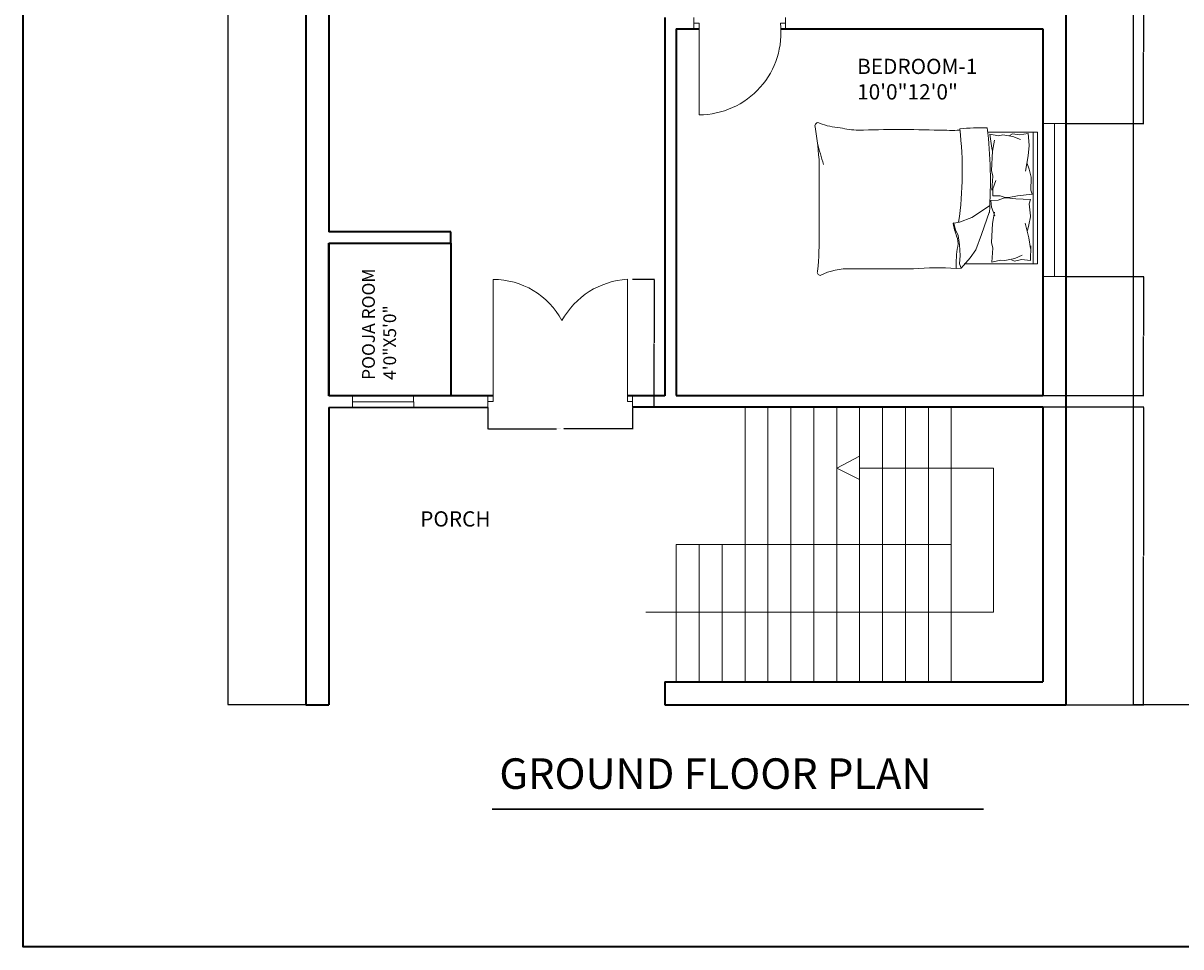
# Model space of a CAD drawing. Units: inches. Extents: x 2416 to 3391, y 1375 to 2496.
# Tile 1 of 13: x 2416 to 2871, y 1375 to 1738. Entities that reach past the tile are written whole.
import ezdxf

# ---------------------------------------------------------------- set-up
doc = ezdxf.new("R2010")
doc.units = ezdxf.units.IN
for name, color, linetype, lineweight in [('A-ANNO-DIMS', 2, 'Continuous', 18), ('A-ANNO-TITL', 7, 'Continuous', 30), ('A-ANNO-TTLB', 7, 'Continuous', 35), ('A-AREA-IDEN', 7, 'Continuous', 18), ('A-DOOR', 3, 'Continuous', 20), ('A-FLOR-STRS', 7, 'Continuous', 20), ('A-FURN', 8, 'Continuous', 18), ('A-GLAZ', 4, 'Continuous', 18), ('A-WALL', 7, 'Continuous', 35)]:
    doc.layers.add(name, color=color, linetype=linetype, lineweight=lineweight)
doc.styles.get("Standard").update_dxf_attribs({"font": 'arial.ttf'})
doc.dimstyles.get("Standard").update_dxf_attribs({"dimtxt": 0.18, "dimasz": 0.18, "dimexe": 0.18, "dimexo": 0.0625, "dimgap": 0.09, "dimtad": 0, "dimtih": 1, "dimtoh": 1, "dimdec": 4, "dimzin": 0, "dimdsep": 46, "dimtxsty": 'Standard', "dimcen": 0.09, "dimadec": 0, "dimazin": 0, "dimtfac": 1, "dimtdec": 4, "dimtofl": 0, "dimtmove": 0, "dimatfit": 3, "dimfxl": 1, "dimtolj": 1, "dimtzin": 0, "dimarcsym": 0})

# ---------------------------------------------------------------- blocks, each defined once
blk = doc.blocks.new('WINDOW-60IN')
for p, q in [((0, 60), (9, 60)), ((9, 60), (4.5, 60)), ((4.5, 60), (4.5, 0)), ((4.5, 0), (0, 0)), ((0, 0), (9, 0))]:
    blk.add_line(p, q)
blk = doc.blocks.new('WINDOW-24IN-INT')
for p, q in [((0, 4.49), (0.01, 0)), ((0.01, 0), (0, 2.24)), ((0, 2.24), (24, 2.24)), ((24, 2.24), (24, 4.49)), ((24, 4.49), (24.01, 0.03))]:
    blk.add_line(p, q)
blk = doc.blocks.new('DOOR-BED-SOUTH')
for p, q in [((-2, 2.25), (-2, -2.25)), ((33.94, 2.25), (33.94, -2.25)), ((-2, -2.25), (-2, 0)), ((-2, 0), (0, 0)), ((0, 0), (0, -36)), ((33.94, 0), (31.94, 0))]:
    blk.add_line(p, q)
blk.add_arc((0, -3.83), 32.17, 270, 6.8343)
blk = doc.blocks.new('DOOR-ENTRY-PAIR')
for p, q in [((0, 0), (0, 48)), ((52.72, 0.04), (52.72, 48.04)), ((-2, 2.21), (-2, -2.21)), ((-2, 0), (0, 0)), ((54.72, 0.04), (52.72, 0.04)), ((54.72, 2.21), (54.73, -2.13)), ((54.73, -2.13), (54.72, 0.04))]:
    blk.add_line(p, q)
for centre, radius, start, end in [((0, 17.33), 30.67, 28.1202, 90), ((54.61, 16.65), 31.45, 93.4374, 151.2249)]:
    blk.add_arc(centre, radius, start, end)
blk = doc.blocks.new('STAIR-RETURN-PLAN')
for p, q in [((27, 0), (27, 108)), ((36, 0), (36, 108)), ((45, 0), (45, 108)), ((54, 0), (54, 108)), ((63, 0), (63, 108)), ((72, 0), (72, 108)), ((81, 0), (81, 108)), ((90, 0), (90, 108)), ((99, 0), (99, 108)), ((108, 0), (108, 108)), ((63, 83.93), (72, 88.71)), ((72, 88.71), (72, 80.54)), ((63, 83.93), (72, 79.53)), ((124.59, 83.93), (72, 83.93)), ((124.59, 27.37), (124.59, 83.93)), ((0, 0), (0, 54)), ((0, 54), (108, 54)), ((9, 0), (9, 54)), ((18, 0), (18, 54)), ((-11.89, 27.37), (124.59, 27.37)), ((-4.5, 0), (0, 0))]:
    blk.add_line(p, q)
blk = doc.blocks.new('BED-PILLOWS-PLAN')
for p, q in [((67.77, 56.25), (87.35, 56.25)), ((69.39, 49.97), (68.6, 55.48)), ((68.6, 55.48), (72.04, 54.86)), ((72.04, 54.86), (73.76, 55.17)), ((73.76, 55.17), (77.67, 54.55)), ((77.51, 55.64), (76.42, 55.02)), ((80.33, 55.17), (77.51, 55.64)), ((83.77, 55.8), (80.33, 55.17)), ((83.74, 55.79), (84.1, 51.16)), ((85.69, 56.25), (85.69, 4.59)), ((87.35, 56.25), (87.35, 4.59)), ((70.46, 53.11), (69.74, 48.75)), ((77.67, 54.55), (80.64, 53.45)), ((84.08, 51.05), (83.77, 46.92)), ((84.1, 51.16), (84.08, 51.05)), ((69.74, 48.75), (69.27, 41.17)), ((69.74, 48.75), (69.39, 49.97)), ((83.77, 46.92), (82.67, 40.98)), ((1.68, 43.72), (1.68, 17.11)), ((69.27, 41.17), (69.87, 39.05)), ((83.3, 43.95), (84.08, 41.76)), ((84.08, 41.76), (84.86, 38.64)), ((69.87, 39.05), (69.44, 33.5)), ((69.77, 33.95), (70.95, 37.35)), ((84.86, 38.29), (84.7, 33.48)), ((84.86, 38.64), (84.86, 38.29)), ((69.77, 31.29), (69.77, 33.95)), ((85.33, 31.92), (79.55, 31.29)), ((84.7, 33.48), (85.33, 31.92)), ((68.56, 27.3), (61.54, 22.77)), ((71.98, 29.6), (69.09, 29.42)), ((69.09, 29.42), (69.25, 26.77)), ((72.67, 31.29), (69.77, 31.29)), ((73.97, 30.35), (71.98, 29.6)), ((74.7, 30.67), (72.67, 31.29)), ((75.38, 30.44), (73.97, 30.35)), ((76.11, 30.67), (74.7, 30.67)), ((78.85, 30.03), (75.38, 30.44)), ((79.55, 31.29), (76.11, 30.67)), ((84.66, 29.76), (78.85, 30.03)), ((84.13, 28.16), (84.66, 29.76)), ((84.59, 23.38), (84.13, 28.16)), ((61.54, 22.77), (56.69, 20.92)), ((65.39, 16.07), (68.56, 25.08)), ((69.25, 26.77), (70.64, 23.45)), ((70.46, 24.8), (69.74, 20.45)), ((84.02, 19.86), (84.61, 23.03)), ((84.61, 23.03), (84.59, 23.38)), ((56.69, 20.92), (54.51, 20.59)), ((54.51, 20.59), (55.18, 17.91)), ((69.74, 20.45), (69.27, 12.87)), ((84.03, 14.7), (82.57, 20.55)), ((83.38, 17.63), (84.02, 19.86)), ((55.18, 17.91), (56.19, 15.73)), ((56.19, 15.73), (56.69, 12.05)), ((63.21, 10.04), (65.39, 16.07)), ((84.6, 10.59), (84.03, 14.7)), ((56.69, 12.05), (57.02, 7.87)), ((60.87, 6.86), (63.21, 10.04)), ((69.27, 12.87), (69.87, 10.75)), ((69.87, 10.75), (69.44, 5.2)), ((84.59, 5.83), (84.69, 11.67)), ((84.69, 11.67), (84.6, 10.59)), ((57.02, 7.87), (56.69, 4.52)), ((57.36, 2.86), (60.87, 6.86)), ((87.35, 4.59), (58.58, 4.59)), ((69.44, 5.2), (72.83, 6.04)), ((72.83, 6.04), (74.56, 5.83)), ((74.56, 5.83), (78.42, 6.7)), ((78.34, 5.6), (77.21, 6.16)), ((81.12, 6.24), (78.34, 5.6)), ((78.42, 6.7), (81.32, 7.98)), ((84.59, 5.83), (81.12, 6.24)), ((55.47, 2.77), (57.36, 2.86, 4.18)), ((56.69, 4.52), (57.36, 2.86))]:
    blk.add_line(p, q)
for centre, radius, start, end in [((1.17, 58.83), 1.18, 56.1736, 203.4781), ((11.38, 83.42), 25.47, 247.9751, 266.652), ((-129.76, 36.84), 131.62, 2.9958, 9.4091), ((17.61, 89.09), 32.04, 256.0648, 268.9113), ((32.64, -464.1), 521.39, 88.2277, 91.7185), ((53.65, 240.87), 183.89, 268.4762, 271.0082), ((-81.63, 40.81), 139.47, 351.7845, 6.9006), ((65.63, -32.06), 90.06, 88.7218, 95.604), ((-109.45, 36.92), 178.34, 356.0865, 6.7821), ((112.98, 78.62), 115.08, 193.3832, 197.7053), ((54.44, 20.4), 0.199, 70.2464, 181.1377), ((85.75, 26.33), 32.06, 190.6617, 199.8806), ((-142.13, 15.52), 143.82, 354.4998, 0.6351), ((49.44, 12.72), 6.73, 348.6608, 23.7384), ((94.55, 4.52), 39.11, 169.8763, 182.5657), ((2.09, 1.19), 1.19, 152.6588, 266.02), ((13.12, -22.32), 24.93, 87.4714, 116.4681), ((14.03, 4934.07), 4931.49, 270.00217, 270.28689), ((48.09, -137.03), 139.99, 86.9791, 93.8365)]:
    blk.add_arc(centre, radius, start, end)
blk = doc.blocks.new('*D35')
at = {"layer": 'A-ANNO-DIMS', "color": 0, "lineweight": -2, "transparency": 16777216}
for p, q in [((2599, 1587.01), (2599, 1578.39)), ((2655.73, 1587.01), (2655.73, 1578.39)), ((2599.18, 1578.57), (2625.89, 1578.57)), ((2655.55, 1578.57), (2628.85, 1578.57))]:
    blk.add_line(p, q, dxfattribs=at)
at = {"layer": 'A-ANNO-DIMS', "color": 0, "transparency": 16777216}
for points in [[(2599.18, 1578.6), (2599.18, 1578.54), (2599, 1578.57)], [(2655.55, 1578.6), (2655.55, 1578.54), (2655.73, 1578.57)]]:
    blk.add_solid(points, dxfattribs=at)
at = {"layer": 'Defpoints', "color": 0, "transparency": 16777216}
for p in [(2599, 1587.08), (2655.73, 1587.08), (2655.73, 1578.57)]:
    blk.add_point(p, dxfattribs=at)
at = {"layer": 'A-ANNO-DIMS', "color": 0, "transparency": 16777216, "insert": (2627.37, 1578.57), "char_height": 0.18, "attachment_point": 5}
blk.add_mtext('\\A1;ENTRY DOORS 57 TYP.', dxfattribs=at)
blk = doc.blocks.new('*D36')
at = {"layer": 'A-ANNO-DIMS', "color": 0, "lineweight": -2, "transparency": 16777216}
for p, q in [((2655.79, 1637.32), (2664.42, 1637.32)), ((2664.24, 1637.14), (2664.24, 1612.38)), ((2664.24, 1587.26), (2664.24, 1612.02)), ((2655.79, 1587.08), (2664.42, 1587.08))]:
    blk.add_line(p, q, dxfattribs=at)
at = {"layer": 'A-ANNO-DIMS', "color": 0, "transparency": 16777216}
for points in [[(2664.21, 1637.14), (2664.27, 1637.14), (2664.24, 1637.32)], [(2664.21, 1587.26), (2664.27, 1587.26), (2664.24, 1587.08)]]:
    blk.add_solid(points, dxfattribs=at)
at = {"layer": 'Defpoints', "color": 0, "transparency": 16777216}
for p in [(2655.73, 1637.32), (2664.24, 1637.32), (2655.73, 1587.08)]:
    blk.add_point(p, dxfattribs=at)
at = {"layer": 'A-ANNO-DIMS', "color": 0, "transparency": 16777216, "insert": (2664.24, 1612.2), "char_height": 0.18, "attachment_point": 5}
blk.add_mtext('\\A1;50 TYP.', dxfattribs=at)
blk = doc.blocks.new('*D48')
at = {"layer": 'A-ANNO-DIMS', "color": 0, "lineweight": -2, "transparency": 16777216}
for p, q in [((2527.38, 2034.17), (2496.81, 2034.17)), ((2496.99, 2033.99), (2496.99, 1752.35)), ((2496.99, 1470.35), (2496.99, 1751.99)), ((2527.38, 1470.17), (2496.81, 1470.17))]:
    blk.add_line(p, q, dxfattribs=at)
at = {"layer": 'A-ANNO-DIMS', "color": 0, "transparency": 16777216}
for points in [[(2496.96, 2033.99), (2497.02, 2033.99), (2496.99, 2034.17)], [(2496.96, 1470.35), (2497.02, 1470.35), (2496.99, 1470.17)]]:
    blk.add_solid(points, dxfattribs=at)
at = {"layer": 'Defpoints', "color": 0, "transparency": 16777216}
for p in [(2496.99, 2034.17), (2527.44, 2034.17), (2527.44, 1470.17)]:
    blk.add_point(p, dxfattribs=at)
at = {"layer": 'A-ANNO-DIMS', "color": 0, "transparency": 16777216, "insert": (2496.99, 1752.17), "char_height": 0.18, "attachment_point": 5}
blk.add_mtext('\\A1;564', dxfattribs=at)
blk = doc.blocks.new('*D49')
at = {"layer": 'A-ANNO-DIMS', "color": 0, "lineweight": -2, "transparency": 16777216}
for p, q in [((2817, 1587.17), (2856.57, 1587.17)), ((2856.39, 1586.99), (2856.39, 1528.85)), ((2856.39, 1470.35), (2856.39, 1528.49)), ((2826, 1470.17), (2856.57, 1470.17))]:
    blk.add_line(p, q, dxfattribs=at)
at = {"layer": 'A-ANNO-DIMS', "color": 0, "transparency": 16777216}
for points in [[(2856.36, 1586.99), (2856.42, 1586.99), (2856.39, 1587.17)], [(2856.36, 1470.35), (2856.42, 1470.35), (2856.39, 1470.17)]]:
    blk.add_solid(points, dxfattribs=at)
at = {"layer": 'Defpoints', "color": 0, "transparency": 16777216}
for p in [(2816.94, 1587.17), (2856.39, 1587.17), (2825.94, 1470.17)]:
    blk.add_point(p, dxfattribs=at)
at = {"layer": 'A-ANNO-DIMS', "color": 0, "transparency": 16777216, "insert": (2856.39, 1528.67), "char_height": 0.18, "attachment_point": 5}
blk.add_mtext('\\A1;117', dxfattribs=at)
blk = doc.blocks.new('*D51')
at = {"layer": 'A-ANNO-DIMS', "color": 0, "lineweight": -2, "transparency": 16777216}
for p, q in [((2826, 1638.45), (2856.57, 1638.45)), ((2856.39, 1638.27), (2856.39, 1615.24)), ((2856.39, 1591.85), (2856.39, 1614.88)), ((2817, 1591.67), (2856.57, 1591.67))]:
    blk.add_line(p, q, dxfattribs=at)
at = {"layer": 'A-ANNO-DIMS', "color": 0, "transparency": 16777216}
for points in [[(2856.36, 1638.27), (2856.42, 1638.27), (2856.39, 1638.45)], [(2856.36, 1591.85), (2856.42, 1591.85), (2856.39, 1591.67)]]:
    blk.add_solid(points, dxfattribs=at)
at = {"layer": 'Defpoints', "color": 0, "transparency": 16777216}
for p in [(2825.94, 1638.45), (2816.94, 1591.67), (2856.39, 1591.67)]:
    blk.add_point(p, dxfattribs=at)
at = {"layer": 'A-ANNO-DIMS', "color": 0, "transparency": 16777216, "insert": (2856.39, 1615.06), "char_height": 0.18, "attachment_point": 5}
blk.add_mtext('\\A1;46.78', dxfattribs=at)
blk = doc.blocks.new('*D52')
at = {"layer": 'A-ANNO-DIMS', "color": 0, "lineweight": -2, "transparency": 16777216}
for p, q in [((2826, 1754.58), (2856.57, 1754.58)), ((2856.39, 1754.4), (2856.39, 1726.7)), ((2856.39, 1698.63), (2856.39, 1726.33)), ((2826, 1698.45), (2856.57, 1698.45))]:
    blk.add_line(p, q, dxfattribs=at)
at = {"layer": 'A-ANNO-DIMS', "color": 0, "transparency": 16777216}
for points in [[(2856.36, 1754.4), (2856.42, 1754.4), (2856.39, 1754.58)], [(2856.36, 1698.63), (2856.42, 1698.63), (2856.39, 1698.45)]]:
    blk.add_solid(points, dxfattribs=at)
at = {"layer": 'Defpoints', "color": 0, "transparency": 16777216}
for p in [(2825.94, 1754.58), (2825.94, 1698.45), (2856.39, 1698.45)]:
    blk.add_point(p, dxfattribs=at)
at = {"layer": 'A-ANNO-DIMS', "color": 0, "transparency": 16777216, "insert": (2856.39, 1726.51), "char_height": 0.18, "attachment_point": 5}
blk.add_mtext('\\A1;56.14', dxfattribs=at)
blk = doc.blocks.new('*D55')
at = {"layer": 'A-ANNO-DIMS', "color": 0, "lineweight": -2, "transparency": 16777216}
for p, q in [((2904.13, 2034.17), (2852.3, 2034.17)), ((2852.48, 2033.99), (2852.48, 1752.35)), ((2852.48, 1470.35), (2852.48, 1751.99)), ((2904.13, 1470.17), (2852.3, 1470.17))]:
    blk.add_line(p, q, dxfattribs=at)
at = {"layer": 'A-ANNO-DIMS', "color": 0, "transparency": 16777216}
for points in [[(2852.45, 2033.99), (2852.51, 2033.99), (2852.48, 2034.17)], [(2852.45, 1470.35), (2852.51, 1470.35), (2852.48, 1470.17)]]:
    blk.add_solid(points, dxfattribs=at)
at = {"layer": 'Defpoints', "color": 0, "transparency": 16777216}
for p in [(2852.48, 2034.17), (2904.19, 2034.17), (2904.19, 1470.17)]:
    blk.add_point(p, dxfattribs=at)
at = {"layer": 'A-ANNO-DIMS', "color": 0, "transparency": 16777216, "insert": (2852.48, 1752.17), "char_height": 0.18, "attachment_point": 5}
blk.add_mtext('\\A1;564', dxfattribs=at)

msp = doc.modelspace()

# ---------------------------------------------------------------- linework, layer by layer
at = {"layer": 'A-ANNO-TITL'}
msp.add_line((2600.6641, 1429.1861), (2793.6466, 1429.1861), dxfattribs=at)
at = {"layer": 'A-ANNO-TTLB'}
msp.add_lwpolyline([(2416.4678, 2496.0939), (3391.2022, 2496.0939), (3391.2022, 1375.1104), (2416.4678, 1375.1104)], close=True, dxfattribs=at)
at = {"layer": 'A-WALL'}
for p, q in [((2527.4424, 2034.17), (2527.4424, 1470.17)), ((2825.9424, 2034.17), (2825.9424, 1470.17)), ((2536.4424, 1936.67), (2536.4424, 1655.9896)), ((2668.4424, 1740.17), (2668.4424, 1591.4896)), ((2672.9424, 1735.67), (2672.9424, 1591.67)), ((2672.9424, 1735.67), (2681.8695, 1735.67)), ((2714.0024, 1735.67), (2816.9424, 1735.67)), ((2816.9424, 1735.67), (2816.9424, 1591.67)), ((2584.4424, 1655.9896), (2536.4424, 1655.9896)), ((2584.4424, 1651.4896), (2584.4424, 1655.9896)), ((2536.4424, 1591.4896), (2536.4424, 1651.4896)), ((2536.4424, 1651.4896), (2584.4424, 1651.4896)), ((2536.4424, 1651.4896), (2536.4424, 1591.4896)), ((2584.4424, 1651.4896), (2584.4424, 1591.4896)), ((2601.0051, 1591.4896), (2536.4424, 1591.4896)), ((2668.4424, 1591.4896), (2653.729, 1591.4896)), ((2672.9424, 1591.67), (2816.9424, 1591.67)), ((2536.4424, 1586.9896), (2599.0081, 1587.0751)), ((2536.4424, 1586.9896), (2536.4424, 1470.17)), ((2655.732, 1587.1527), (2668.4424, 1587.17)), ((2668.4424, 1587.17), (2816.9424, 1587.17)), ((2816.9424, 1587.17), (2816.9424, 1479.17)), ((2668.4424, 1479.17), (2816.9424, 1479.17)), ((2668.4424, 1479.17), (2668.4424, 1470.17)), ((2527.4424, 1470.17), (2536.4424, 1470.17)), ((2668.4424, 1470.17), (2825.9424, 1470.17))]:
    msp.add_line(p, q, dxfattribs=at)

# ---------------------------------------------------------------- block references
at = {"layer": 'A-DOOR'}
for name, p in [('DOOR-BED-SOUTH', (2681.8695, 1737.92)), ('DOOR-ENTRY-PAIR', (2601.0051, 1589.2824))]:
    msp.add_blockref(name, p, dxfattribs=at)
at = {"layer": 'A-FLOR-STRS'}
msp.add_blockref('STAIR-RETURN-PLAN', (2672.9424, 1479.17), dxfattribs=at)
at = {"layer": 'A-FURN'}
msp.add_blockref('BED-PILLOWS-PLAN', (2727.4194, 1638.8314), dxfattribs=at)
at = {"layer": 'A-GLAZ'}
for name, p in [('WINDOW-60IN', (2816.942, 1638.4452)), ('WINDOW-24IN-INT', (2545.812, 1587.002))]:
    msp.add_blockref(name, p, dxfattribs=at)

# ---------------------------------------------------------------- texts
at = {"layer": 'A-ANNO-TITL', "insert": (2603.4679, 1449.1546), "char_height": 12, "attachment_point": 1}
msp.add_mtext_dynamic_manual_height_columns('GROUND FLOOR PLAN', width=195.734447, gutter_width=12.5, heights=[0], dxfattribs=at)
at = {"layer": 'A-AREA-IDEN', "char_height": 6, "attachment_point": 1}
for s, width, insert in [('BEDROOM-1\\P10\'0"12\'0"', 77.663477, (2743.9483, 1723.9353)), ('PORCH', 244.556397, (2572.386, 1546.1894))]:
    msp.add_mtext_dynamic_manual_height_columns(s, width=width, gutter_width=12.5, heights=[0], dxfattribs=dict(at, insert=insert))
at = {"layer": 'A-AREA-IDEN', "insert": (2549.5735, 1597.7958), "char_height": 5, "attachment_point": 1, "rotation": 90}
msp.add_mtext_dynamic_manual_height_columns('POOJA ROOM\\P4\'0"X5\'0"', width=78.872259, gutter_width=12.5, heights=[0], dxfattribs=at)

# ---------------------------------------------------------------- dimensions: what is measured, and where the dimension line sits
at = {"layer": 'A-ANNO-DIMS'}
for base, p1, p2, override, picture, middle in [((2496.9924, 2034.17), (2527.4424, 1470.17), (2527.4424, 2034.17), {"dimdec": 0, "dimlfac": 1, "dimrnd": 0, "dimzin": 0, "dimdsep": 46, "dimlunit": 2}, '*D48', (2496.9924, 1752.17)), ((2852.4781, 2034.17), (2904.1924, 1470.17), (2904.1924, 2034.17), {"dimdec": 0, "dimlfac": 1, "dimrnd": 0, "dimzin": 0, "dimdsep": 46, "dimlunit": 2}, '*D55', (2852.4781, 1752.17)), ((2856.3924, 1698.4455), (2825.9424, 1754.5813), (2825.9424, 1698.4455), {"dimdec": 2, "dimlfac": 1, "dimrnd": 0, "dimzin": 0, "dimdsep": 46, "dimlunit": 2}, '*D52', (2856.3924, 1726.5134)), ((2856.3924, 1591.67), (2825.9424, 1638.4455), (2816.9424, 1591.67), {"dimdec": 2, "dimlfac": 1, "dimrnd": 0, "dimzin": 0, "dimdsep": 46, "dimlunit": 2}, '*D51', (2856.3924, 1615.0578)), ((2856.3924, 1587.17), (2825.9424, 1470.17), (2816.9424, 1587.17), {"dimdec": 0, "dimlfac": 1, "dimrnd": 0, "dimzin": 0, "dimdsep": 46, "dimlunit": 2}, '*D49', (2856.3924, 1528.67))]:
    dim = msp.add_linear_dim(base=base, p1=p1, p2=p2, angle=90, dimstyle='Standard', override=override, dxfattribs=at)
    dim.commit()
    dim.dimension.update_dxf_attribs({"geometry": picture, "text_midpoint": middle})
dim = msp.add_linear_dim(base=(2664.2415, 1637.3211), p1=(2655.732, 1587.0751), p2=(2655.732, 1637.3211), angle=90, text='<> TYP.', dimstyle='Standard', override={"dimdec": 0, "dimlfac": 1, "dimrnd": 0, "dimzin": 0, "dimdsep": 46, "dimlunit": 2}, dxfattribs=at)
dim.commit()
dim.dimension.update_dxf_attribs({"geometry": '*D36', "text_midpoint": (2664.2415, 1612.1981)})
dim = msp.add_linear_dim(base=(2655.732, 1578.5657), p1=(2599.0021, 1587.0751), p2=(2655.732, 1587.0751), text='ENTRY DOORS <> TYP.', dimstyle='Standard', override={"dimdec": 0, "dimlfac": 1, "dimrnd": 0, "dimzin": 0, "dimdsep": 46, "dimlunit": 2}, dxfattribs=at)
dim.commit()
dim.dimension.update_dxf_attribs({"geometry": '*D35', "text_midpoint": (2627.367, 1578.5657)})

doc.saveas('drawing.dxf')
